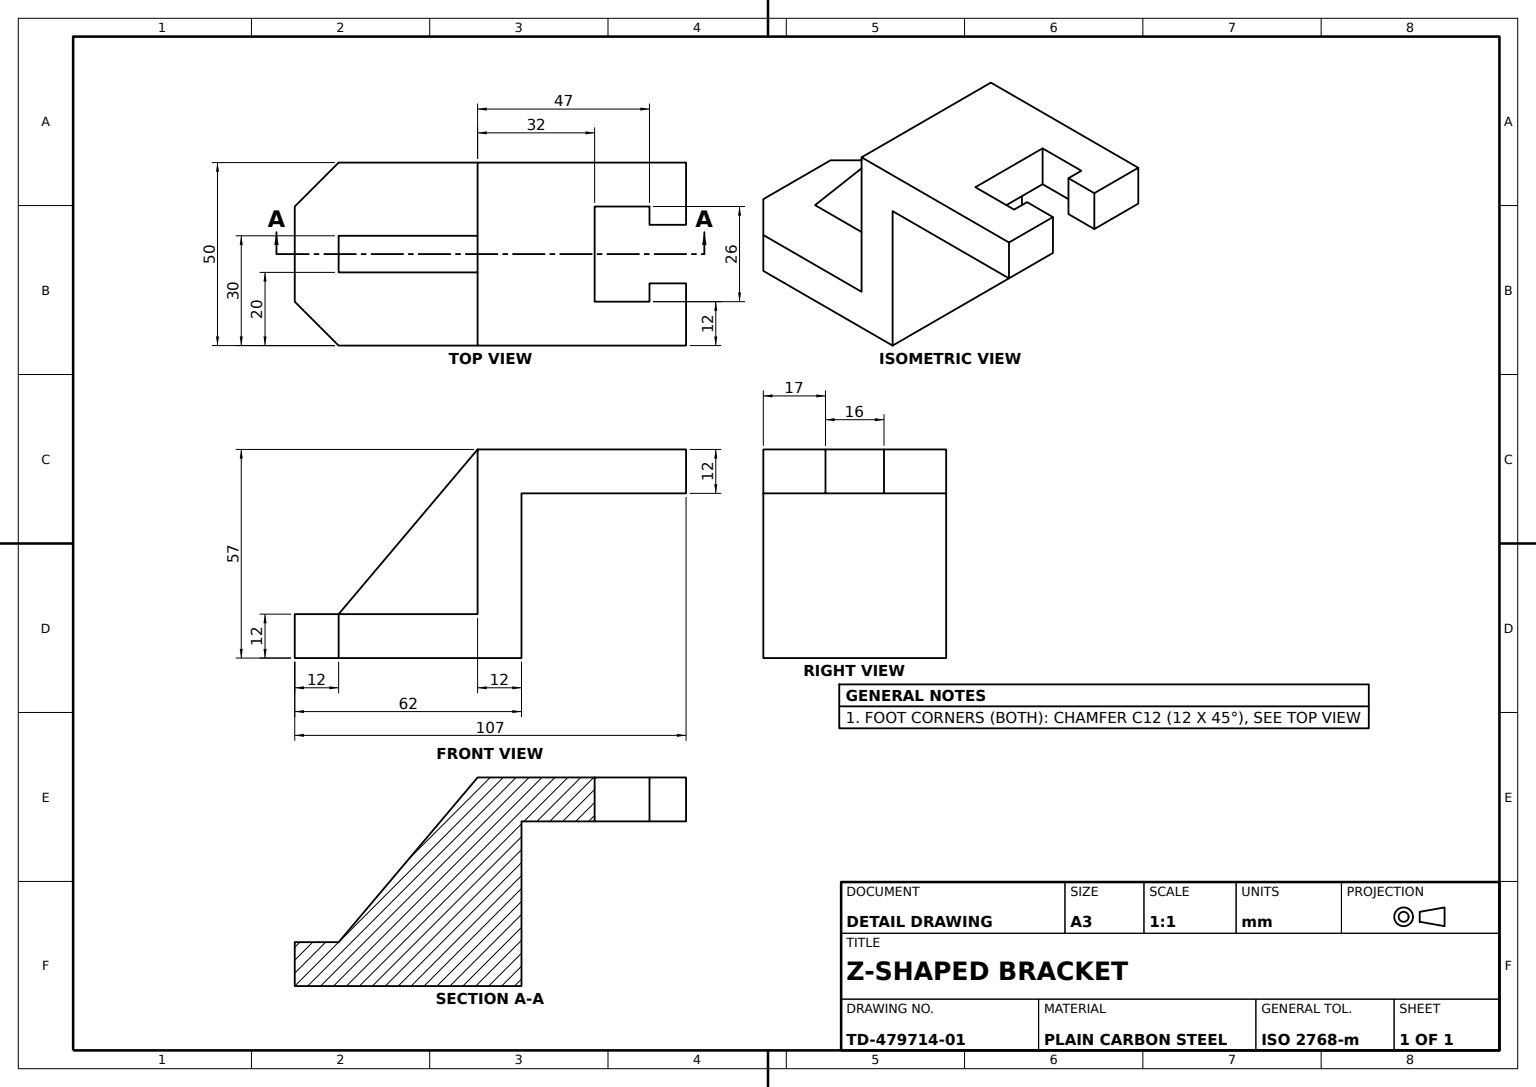
SolidWorks part; units mm, degrees
material "Plain Carbon Steel"
ref_plane "Front Plane" through (0, 0, 0) normal (0, 0, 1) x (1, 0, 0)
ref_plane "Top Plane" through (0, 0, 0) normal (0, 1, 0) x (1, 0, 0)
ref_plane "Right Plane" through (0, 0, 0) normal (1, 0, 0) x (0, 0, -1)
sketch "Bracket Body Profile" plane through (0, 0, 0) normal (0, 0, 1) x (1, 0, 0)
  line L0 (0, 0) -> (12, 0)
  line L1 (12, 0) -> (62, 0)
  line L2 (62, 0) -> (62, 45)
  line L3 (62, 45) -> (107, 45)
  line L5 (0, 0) -> (0, 12)
  line L6 (0, 12) -> (12, 12)
  line L8 (12, 12) -> (50, 12)
  line L9 (107, 45) -> (107, 57)
  line L10 (107, 57) -> (50, 57)
  line L11 (50, 57) -> (50, 12)
  dimension "D1" = 12
  dimension "D2" = 50
  dimension "D3" = 62
  dimension "D4" = 107
extrude "Bracket Body 50mm" add sketch "Bracket Body Profile" along normal blind 50
sketch "Step Pocket Profile" plane through (0, 12, 0) normal (0, 1, 0) x (1, 0, 0)
  line L0 (0, -12) -> (0, 0)
  line L1 (50, 0) -> (0, 0) construction
  line L4 (0, -50) -> (0, 0) construction
  line L5 (0, -12) -> (12, 0)
  line L6 (0, 0) -> (12, 0)
  line L7 (0, -50) -> (0, -38)
  line L8 (0, -50) -> (12, -50)
  line L9 (50, -50) -> (0, -50) construction
  line L10 (12, -50) -> (0, -38)
  dimension "D1" = 12
extrude "Step Pocket 12mm" cut sketch "Step Pocket Profile" against normal blind 12
sketch "Slot Cut Profile" plane through (0, 57, 0) normal (0, 1, 0) x (1, 0, 0)
  line L0 (107, -25) -> (107, -17)
  line L1 (107, -50) -> (107, 0) construction
  line L2 (107, -17) -> (97, -17)
  line L3 (107, -25) -> (107, -33)
  line L4 (107, -33) -> (97, -33)
  line L5 (97, -33) -> (97, -38)
  line L6 (97, -38) -> (82, -38)
  line L7 (82, -38) -> (82, -12)
  line L8 (82, -12) -> (97, -12)
  line L9 (97, -12) -> (97, -17)
  line L10 (50, -50) -> (50, 0) construction
  line L11 (107, 0) -> (50, 0) construction
  dimension "D1" = 32
  dimension "D2" = 47
  dimension "D3" = 12
  dimension "D4" = 17
extrude "Slot Cut 12mm" cut sketch "Slot Cut Profile" against normal blind 12
sketch "Triangular Boss Profile" plane through (0, 0, 50) normal (0, 0, 1) x (1, 0, 0)
  line L0 (12, 12) -> (50, 12)
  line L1 (50, 12) -> (50, 57)
  line L2 (50, 57) -> (12, 12)
extrude "Triangular Boss 30mm" add sketch "Triangular Boss Profile" against normal blind 30
sketch "Triangular Cut Profile" plane through (0, 0, 50) normal (0, 0, 1) x (1, 0, 0)
  line L0 (12, 12) -> (50, 57)
  line L1 (50, 57) -> (50, 12)
  line L2 (50, 12) -> (12, 12)
extrude "Triangular Cut 20mm" cut sketch "Triangular Cut Profile" against normal blind 20
